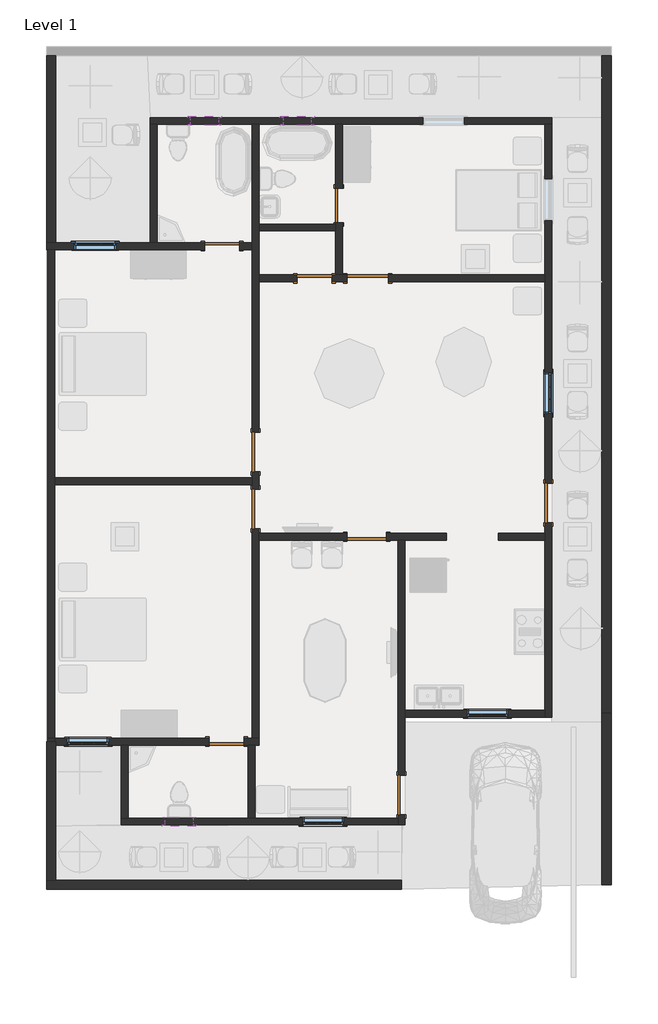
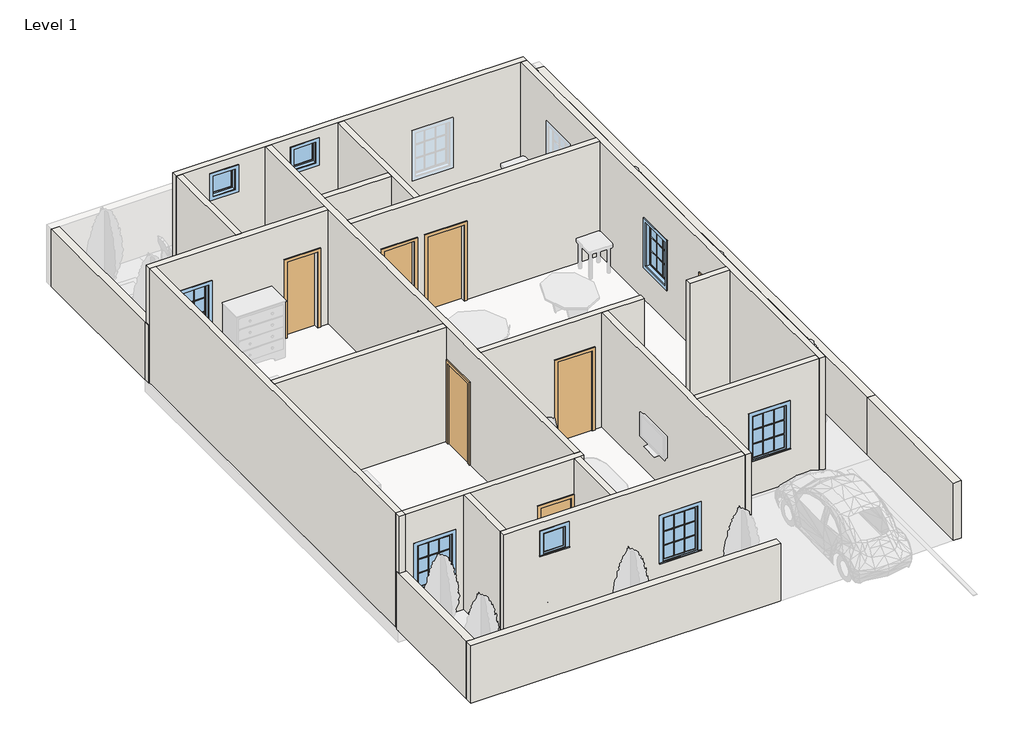
# One storey, part 1 of 2: 24 walls, 10 doors, 8 windows.
"""IFC4 building model written with IfcOpenShell, lengths in millimetres."""

from ifc_helpers import new_model, si_unit, frame, origin, origin_with_axes, place, context, project, spatial, polyline, outline, extrude, faceted_brep, transform, mapped, element, save
from components import door_059fdd7e, door_255cab33, door_99d96fc5, door_b6e9fca3, door_2b0b55a0, window_5c190c7e, window_3d781103

model = new_model("IFC4")

# Units and contexts
model_context = context("Model", 3, world=origin())
ifc_project = project(units=[si_unit("LENGTHUNIT", "METRE", prefix="MILLI")], contexts=[model_context])

# Site, building, storey
site = spatial("IfcSite", under=ifc_project)
building = spatial("IfcBuilding", under=site)
storey = spatial("IfcBuildingStorey", under=building, Name="Level 1", Elevation=0.0)

# Doors
placement = place(None, origin())
door_shape = door_059fdd7e(model_context)
element("IfcDoor", 1, ObjectType="Single-Flush : 30\" x 80\"", at=placement, inside=storey, context=model_context, shape_type="MappedRepresentation", body=[
    mapped(door_shape, transform((-11969.0159934, 7134.0673329, 0.0), x_axis=(1.0, 0.0, 0.0), y_axis=(0.0, 1.0, 0.0), z_axis=(0.0, 0.0, 1.0))),
])
element("IfcDoor", 2, ObjectType="Single-Flush : 30\" x 80\"", at=placement, inside=storey, context=model_context, shape_type="MappedRepresentation", body=[
    mapped(door_shape, transform((-9937.0159934, 6422.8673329, 0.0), x_axis=(1.0, 0.0, 0.0), y_axis=(0.0, 1.0, 0.0), z_axis=(0.0, 0.0, 1.0))),
])
door_2_shape = door_255cab33(model_context)
element("IfcDoor", 3, ObjectType="Single-Flush : 30\" x 80\"", at=placement, inside=storey, context=model_context, shape_type="MappedRepresentation", body=[
    mapped(door_2_shape, transform((-9403.6159934, 8023.0673329, 0.0), x_axis=(0.0, -1.0, 0.0), y_axis=(1.0, 0.0, 0.0), z_axis=(0.0, 0.0, 1.0))),
])
element("IfcDoor", 4, ObjectType="Single-Flush : 30\" x 80\"", at=placement, inside=storey, context=model_context, shape_type="MappedRepresentation", body=[
    mapped(door_2_shape, transform((-11867.4159934, -3737.1326671, 0.0), x_axis=(1.0, 0.0, 0.0), y_axis=(0.0, 1.0, 0.0), z_axis=(0.0, 0.0, 1.0))),
])
door_3_shape = door_99d96fc5(model_context)
element("IfcDoor", 5, ObjectType="Single-Flush : 34\" x 84\"", at=placement, inside=storey, context=model_context, shape_type="MappedRepresentation", body=[
    mapped(door_3_shape, transform((-11232.4159934, 2612.8673329, 0.0), x_axis=(0.0, -1.0, 0.0), y_axis=(1.0, 0.0, 0.0), z_axis=(0.0, 0.0, 1.0))),
])
element("IfcDoor", 6, ObjectType="Single-Flush : 34\" x 84\"", at=placement, inside=storey, context=model_context, shape_type="MappedRepresentation", body=[
    mapped(door_3_shape, transform((-4806.2159934, 1495.2673329, 0.0), x_axis=(0.0, -1.0, 0.0), y_axis=(1.0, 0.0, 0.0), z_axis=(0.0, 0.0, 1.0))),
])
element("IfcDoor", 7, ObjectType="Single-Flush : 34\" x 84\"", at=placement, inside=storey, context=model_context, shape_type="MappedRepresentation", body=[
    mapped(door_3_shape, transform((-8794.0159934, 758.6673329, 0.0), x_axis=(1.0, 0.0, 0.0), y_axis=(0.0, 1.0, 0.0), z_axis=(0.0, 0.0, 1.0))),
])
element("IfcDoor", 8, ObjectType="Single-Flush : 34\" x 84\"", at=placement, inside=storey, context=model_context, shape_type="MappedRepresentation", body=[
    mapped(door_3_shape, transform((-8032.0159934, -4905.5326671, 0.0), x_axis=(0.0, -1.0, 0.0), y_axis=(1.0, 0.0, 0.0), z_axis=(0.0, 0.0, 1.0))),
])
door_4_shape = door_b6e9fca3(model_context)
element("IfcDoor", 9, ObjectType="Single-Flush : 34\" x 84\"", at=placement, inside=storey, context=model_context, shape_type="MappedRepresentation", body=[
    mapped(door_4_shape, transform((-11232.4159934, 1368.2673329, 0.0), x_axis=(0.0, 1.0, 0.0), y_axis=(-1.0, 0.0, 0.0), z_axis=(0.0, 0.0, 1.0))),
])
door_5_shape = door_2b0b55a0(model_context)
element("IfcDoor", 10, ObjectType="Single-Flush : 36\" x 80\"", at=placement, inside=storey, context=model_context, shape_type="MappedRepresentation", body=[
    mapped(door_5_shape, transform((-8768.6159934, 6422.8673329, 0.0), x_axis=(-1.0, 0.0, 0.0), y_axis=(0.0, -1.0, 0.0), z_axis=(0.0, 0.0, 1.0))),
])

# Walls
element("IfcWall", 11, ObjectType="Generic - 8\"", at=placement, inside=storey, context=model_context, shape_type="SweptSolid", body=[
    extrude(outline(polyline([(-3629.9727047, -3120.0940071), (-3629.9727047, 11307.1059929), (-3426.7727047, 11307.1059929), (-3426.7727047, -3120.0940071), (-3629.9727047, -3120.0940071)])), origin_with_axes(), (0.0, 0.0, 1.0), 1524.0),
])
element("IfcWall", 12, ObjectType="Generic - 8\"", at=placement, inside=storey, context=model_context, shape_type="Brep", body=[
    faceted_brep([(-15618.7727047, -6777.6940071, 0.0), (-15618.7727047, -3813.3326671, 0.0), (-15618.7727047, -3737.1326671, 0.0), (-15618.7727047, -3737.1326671, 1524.0), (-15618.7727047, -3813.3326671, 1524.0), (-15618.7727047, -6777.6940071, 1524.0), (-15821.9727047, -6777.6940071, 0.0), (-15821.9727047, -6777.6940071, 1524.0), (-15821.9727047, -3737.1326671, 1524.0), (-15821.9727047, -3737.1326671, 0.0), (-15796.5727047, -3737.1326671, 0.0), (-15644.1727047, -3737.1326671, 0.0), (-15796.5727047, -3737.1326671, 1524.0), (-15644.1727047, -3737.1326671, 1524.0)], [[[0, 1, 2, 3, 4, 5]], [[6, 7, 8, 9]], [[2, 1, 0, 6, 9, 10, 11]], [[3, 2, 11, 10, 9, 8, 12, 13]], [[5, 4, 3, 13, 12, 8, 7]], [[0, 5, 7, 6]]]),
])
element("IfcWall", 13, ObjectType="Generic - 8\"", at=placement, inside=storey, context=model_context, shape_type="Brep", body=[
    faceted_brep([(-15618.7727047, 7210.2673329, 0.0), (-15618.7727047, 11307.1059929, 0.0), (-15618.7727047, 11307.1059929, 1524.0), (-15618.7727047, 7210.2673329, 1524.0), (-15821.9727047, 7210.2673329, 0.0), (-15821.9727047, 7210.2673329, 1524.0), (-15821.9727047, 11307.1059929, 1524.0), (-15821.9727047, 11307.1059929, 0.0), (-15796.5727047, 7210.2673329, 1524.0)], [[[0, 1, 2, 3]], [[4, 5, 6, 7]], [[1, 0, 4, 7]], [[3, 2, 6, 5, 8]], [[2, 1, 7, 6]], [[0, 3, 8, 5, 4]]]),
])
element("IfcWall", 14, ObjectType="Generic - 8\"", at=placement, inside=storey, context=model_context, shape_type="SweptSolid", body=[
    extrude(outline(polyline([(-3629.9727047, -6879.2940071), (-3629.9727047, -3120.0940071), (-3426.7727047, -3120.0940071), (-3426.7727047, -6879.2940071), (-3629.9727047, -6879.2940071)])), origin_with_axes(), (0.0, 0.0, 1.0), 1524.0),
])
element("IfcWall", 15, ObjectType="Generic - 8\"", at=placement, inside=storey, context=model_context, shape_type="Brep", body=[
    faceted_brep([(-8032.0159934, -6777.6940071, 0.0), (-15618.7727047, -6777.6940071, 0.0), (-15821.9727047, -6777.6940071, 0.0), (-15821.9727047, -6777.6940071, 1524.0), (-15618.7727047, -6777.6940071, 1524.0), (-8032.0159934, -6777.6940071, 1524.0), (-8032.0159934, -6980.8940071, 0.0), (-8032.0159934, -6980.8940071, 1524.0), (-15821.9727047, -6980.8940071, 1524.0), (-15821.9727047, -6980.8940071, 0.0)], [[[0, 1, 2, 3, 4, 5]], [[6, 7, 8, 9]], [[2, 1, 0, 6, 9]], [[5, 4, 3, 8, 7]], [[0, 5, 7, 6]], [[3, 2, 9, 8]]]),
])
element("IfcWall", 16, ObjectType="INNER 6\"", at=placement, inside=storey, context=model_context, shape_type="Brep", body=[
    faceted_brep([(-4730.0159934, 9953.4673329, 0.0), (-13543.8159934, 9953.4673329, 0.0), (-13543.8159934, 9953.4673329, 3048.0), (-4730.0159934, 9953.4673329, 3048.0), (-12045.2159934, 9953.4673329, 2768.6), (-12654.8159934, 9953.4673329, 2768.6), (-12654.8159934, 9953.4673329, 2159.0), (-12045.2159934, 9953.4673329, 2159.0), (-10013.2159934, 9953.4673329, 2768.6), (-10622.8159934, 9953.4673329, 2768.6), (-10622.8159934, 9953.4673329, 2159.0), (-10013.2159934, 9953.4673329, 2159.0), (-6647.7159934, 9953.4673329, 2133.6), (-7562.1159934, 9953.4673329, 2133.6), (-7562.1159934, 9953.4673329, 914.4), (-6647.7159934, 9953.4673329, 914.4), (-4730.0159934, 9801.0673329, 0.0), (-4730.0159934, 9801.0673329, 3048.0), (-4882.4159934, 9801.0673329, 3048.0), (-9327.4159934, 9801.0673329, 3048.0), (-9479.8159934, 9801.0673329, 3048.0), (-11156.2159934, 9801.0673329, 3048.0), (-11308.6159934, 9801.0673329, 3048.0), (-13391.4159934, 9801.0673329, 3048.0), (-13543.8159934, 9801.0673329, 3048.0), (-13543.8159934, 9801.0673329, 0.0), (-13391.4159934, 9801.0673329, 0.0), (-11308.6159934, 9801.0673329, 0.0), (-11156.2159934, 9801.0673329, 0.0), (-9479.8159934, 9801.0673329, 0.0), (-9327.4159934, 9801.0673329, 0.0), (-4882.4159934, 9801.0673329, 0.0), (-12045.2159934, 9801.0673329, 2768.6), (-12045.2159934, 9801.0673329, 2159.0), (-12654.8159934, 9801.0673329, 2159.0), (-12654.8159934, 9801.0673329, 2768.6), (-10013.2159934, 9801.0673329, 2768.6), (-10013.2159934, 9801.0673329, 2159.0), (-10622.8159934, 9801.0673329, 2159.0), (-10622.8159934, 9801.0673329, 2768.6), (-6647.7159934, 9801.0673329, 2133.6), (-6647.7159934, 9801.0673329, 914.4), (-7562.1159934, 9801.0673329, 914.4), (-7562.1159934, 9801.0673329, 2133.6)], [[[0, 1, 2, 3], [4, 5, 6, 7], [8, 9, 10, 11], [12, 13, 14, 15]], [[16, 17, 18, 19, 20, 21, 22, 23, 24, 25, 26, 27, 28, 29, 30, 31], [32, 33, 34, 35], [36, 37, 38, 39], [40, 41, 42, 43]], [[1, 0, 16, 31, 30, 29, 28, 27, 26, 25]], [[2, 1, 25, 24]], [[0, 3, 17, 16]], [[33, 32, 4, 7]], [[34, 33, 7, 6]], [[35, 34, 6, 5]], [[32, 35, 5, 4]], [[37, 36, 8, 11]], [[38, 37, 11, 10]], [[39, 38, 10, 9]], [[36, 39, 9, 8]], [[41, 40, 12, 15]], [[42, 41, 15, 14]], [[43, 42, 14, 13]], [[40, 43, 13, 12]], [[3, 2, 24, 23, 22, 21, 20, 19, 18, 17]]]),
])
element("IfcWall", 17, ObjectType="INNER 6\"", at=placement, inside=storey, context=model_context, shape_type="SweptSolid", body=[
    extrude(outline(polyline([(-13543.8159934, 7210.2673329), (-13543.8159934, 9801.0673329), (-13391.4159934, 9801.0673329), (-13391.4159934, 7210.2673329), (-13543.8159934, 7210.2673329)])), origin_with_axes(), (0.0, 0.0, 1.0), 3048.0),
])
element("IfcWall", 18, ObjectType="INNER 6\"", at=placement, inside=storey, context=model_context, shape_type="Brep", body=[
    faceted_brep([(-11308.6159934, 7210.2673329, 0.0), (-11588.0159934, 7210.2673329, 0.0), (-11588.0159934, 7210.2673329, 2032.0), (-12350.0159934, 7210.2673329, 2032.0), (-12350.0159934, 7210.2673329, 0.0), (-13391.4159934, 7210.2673329, 0.0), (-13543.8159934, 7210.2673329, 0.0), (-15618.7727047, 7210.2673329, 0.0), (-15821.9727047, 7210.2673329, 0.0), (-15821.9727047, 7210.2673329, 1524.0), (-15796.5727047, 7210.2673329, 1524.0), (-15796.5727047, 7210.2673329, 3048.0), (-13543.8159934, 7210.2673329, 3048.0), (-13391.4159934, 7210.2673329, 3048.0), (-11308.6159934, 7210.2673329, 3048.0), (-14297.9727047, 7210.2673329, 2133.6), (-15212.3727047, 7210.2673329, 2133.6), (-15212.3727047, 7210.2673329, 914.4), (-14297.9727047, 7210.2673329, 914.4), (-11588.0159934, 7057.8673329, 2032.0), (-11588.0159934, 7057.8673329, 0.0), (-11308.6159934, 7057.8673329, 0.0), (-11308.6159934, 7057.8673329, 3048.0), (-15644.1727047, 7057.8673329, 3048.0), (-15796.5727047, 7057.8673329, 3048.0), (-15796.5727047, 7057.8673329, 1524.0), (-15821.9727047, 7057.8673329, 1524.0), (-15821.9727047, 7057.8673329, 0.0), (-15796.5727047, 7057.8673329, 0.0), (-15644.1727047, 7057.8673329, 0.0), (-12350.0159934, 7057.8673329, 0.0), (-12350.0159934, 7057.8673329, 2032.0), (-14297.9727047, 7057.8673329, 2133.6), (-14297.9727047, 7057.8673329, 914.4), (-15212.3727047, 7057.8673329, 914.4), (-15212.3727047, 7057.8673329, 2133.6)], [[[0, 1, 2, 3, 4, 5, 6, 7, 8, 9, 10, 11, 12, 13, 14], [15, 16, 17, 18]], [[19, 20, 21, 22, 23, 24, 25, 26, 27, 28, 29, 30, 31], [32, 33, 34, 35]], [[21, 20, 1, 0]], [[30, 29, 28, 27, 8, 7, 6, 5, 4]], [[0, 14, 22, 21]], [[2, 1, 20, 19]], [[3, 2, 19, 31]], [[4, 3, 31, 30]], [[33, 32, 15, 18]], [[34, 33, 18, 17]], [[35, 34, 17, 16]], [[32, 35, 16, 15]], [[25, 10, 9, 26]], [[9, 8, 27, 26]], [[11, 10, 25, 24]], [[14, 13, 12, 11, 24, 23, 22]]]),
])
element("IfcWall", 19, ObjectType="INNER 6\"", at=placement, inside=storey, context=model_context, shape_type="Brep", body=[
    faceted_brep([(-4882.4159934, 1063.4673329, 2133.6), (-4882.4159934, 1063.4673329, 0.0), (-4882.4159934, 834.8673329, 0.0), (-4882.4159934, 682.4673329, 0.0), (-4882.4159934, -3051.3326671, 0.0), (-4882.4159934, -3203.7326671, 0.0), (-4882.4159934, -3203.7326671, 3048.0), (-4882.4159934, -3051.3326671, 3048.0), (-4882.4159934, 682.4673329, 3048.0), (-4882.4159934, 834.8673329, 3048.0), (-4882.4159934, 6346.6673329, 3048.0), (-4882.4159934, 6499.0673329, 3048.0), (-4882.4159934, 9801.0673329, 3048.0), (-4882.4159934, 9801.0673329, 0.0), (-4882.4159934, 6499.0673329, 0.0), (-4882.4159934, 6346.6673329, 0.0), (-4882.4159934, 1927.0673329, 0.0), (-4882.4159934, 1927.0673329, 2133.6), (-4882.4159934, 7692.8673329, 2133.6), (-4882.4159934, 7692.8673329, 914.4), (-4882.4159934, 8607.2673329, 914.4), (-4882.4159934, 8607.2673329, 2133.6), (-4882.4159934, 3451.0673329, 2133.6), (-4882.4159934, 3451.0673329, 914.4), (-4882.4159934, 4365.4673329, 914.4), (-4882.4159934, 4365.4673329, 2133.6), (-4730.0159934, -3203.7326671, 0.0), (-4730.0159934, 1063.4673329, 0.0), (-4730.0159934, 1063.4673329, 2133.6), (-4730.0159934, 1927.0673329, 2133.6), (-4730.0159934, 1927.0673329, 0.0), (-4730.0159934, 9801.0673329, 0.0), (-4730.0159934, 9801.0673329, 3048.0), (-4730.0159934, -3203.7326671, 3048.0), (-4730.0159934, 7692.8673329, 2133.6), (-4730.0159934, 8607.2673329, 2133.6), (-4730.0159934, 8607.2673329, 914.4), (-4730.0159934, 7692.8673329, 914.4), (-4730.0159934, 3451.0673329, 2133.6), (-4730.0159934, 4365.4673329, 2133.6), (-4730.0159934, 4365.4673329, 914.4), (-4730.0159934, 3451.0673329, 914.4)], [[[0, 1, 2, 3, 4, 5, 6, 7, 8, 9, 10, 11, 12, 13, 14, 15, 16, 17], [18, 19, 20, 21], [22, 23, 24, 25]], [[26, 27, 28, 29, 30, 31, 32, 33], [34, 35, 36, 37], [38, 39, 40, 41]], [[5, 4, 3, 2, 1, 27, 26]], [[16, 15, 14, 13, 31, 30]], [[13, 12, 32, 31]], [[6, 5, 26, 33]], [[28, 27, 1, 0]], [[29, 28, 0, 17]], [[30, 29, 17, 16]], [[19, 18, 34, 37]], [[20, 19, 37, 36]], [[21, 20, 36, 35]], [[18, 21, 35, 34]], [[23, 22, 38, 41]], [[24, 23, 41, 40]], [[25, 24, 40, 39]], [[22, 25, 39, 38]], [[12, 11, 10, 9, 8, 7, 6, 33, 32]]]),
])
element("IfcWall", 20, ObjectType="INNER 6\"", at=placement, inside=storey, context=model_context, shape_type="SweptSolid", body=[
    extrude(outline(polyline([(0.0, -4882.4159934), (3048.0, -4882.4159934), (3048.0, -7955.8159934), (0.0, -7955.8159934), (0.0, -4882.4159934)]), holes=[polyline([(2133.6, -6596.9159934), (2133.6, -5682.5159934), (914.4, -5682.5159934), (914.4, -6596.9159934), (2133.6, -6596.9159934)])]), frame((0.0, -3203.7326671, 0.0), z_axis=(0.0, 1.0, 0.0), x_axis=(0.0, 0.0, 1.0)), (0.0, 0.0, 1.0), 152.4),
])
element("IfcWall", 21, ObjectType="INNER 6\"", at=placement, inside=storey, context=model_context, shape_type="Brep", body=[
    faceted_brep([(-8108.2159934, -5337.3326671, 2133.6), (-8108.2159934, -5337.3326671, 0.0), (-8108.2159934, -5413.5326671, 0.0), (-8108.2159934, -5565.9326671, 0.0), (-8108.2159934, -5565.9326671, 3048.0), (-8108.2159934, -5413.5326671, 3048.0), (-8108.2159934, 682.4673329, 3048.0), (-8108.2159934, 682.4673329, 0.0), (-8108.2159934, -4473.7326671, 0.0), (-8108.2159934, -4473.7326671, 2133.6), (-7955.8159934, -5565.9326671, 0.0), (-7955.8159934, -5337.3326671, 0.0), (-7955.8159934, -5337.3326671, 2133.6), (-7955.8159934, -4473.7326671, 2133.6), (-7955.8159934, -4473.7326671, 0.0), (-7955.8159934, -3203.7326671, 0.0), (-7955.8159934, -3051.3326671, 0.0), (-7955.8159934, 682.4673329, 0.0), (-7955.8159934, 682.4673329, 3048.0), (-7955.8159934, -3051.3326671, 3048.0), (-7955.8159934, -3203.7326671, 3048.0), (-7955.8159934, -5565.9326671, 3048.0)], [[[0, 1, 2, 3, 4, 5, 6, 7, 8, 9]], [[10, 11, 12, 13, 14, 15, 16, 17, 18, 19, 20, 21]], [[8, 7, 17, 16, 15, 14]], [[3, 2, 1, 11, 10]], [[4, 3, 10, 21]], [[7, 6, 18, 17]], [[12, 11, 1, 0]], [[13, 12, 0, 9]], [[14, 13, 9, 8]], [[6, 5, 4, 21, 20, 19, 18]]]),
])
element("IfcWall", 22, ObjectType="INNER 6\"", at=placement, inside=storey, context=model_context, shape_type="Brep", body=[
    faceted_brep([(-8108.2159934, -5413.5326671, 0.0), (-11246.0185546, -5413.5326671, 0.0), (-11398.4185546, -5413.5326671, 0.0), (-14026.4159934, -5413.5326671, 0.0), (-14178.8159934, -5413.5326671, 0.0), (-14178.8159934, -5413.5326671, 3048.0), (-14026.4159934, -5413.5326671, 3048.0), (-11398.4185546, -5413.5326671, 3048.0), (-11246.0185546, -5413.5326671, 3048.0), (-8108.2159934, -5413.5326671, 3048.0), (-13213.6159934, -5413.5326671, 2768.6), (-13213.6159934, -5413.5326671, 2159.0), (-12604.0159934, -5413.5326671, 2159.0), (-12604.0159934, -5413.5326671, 2768.6), (-10204.6185546, -5413.5326671, 2133.6), (-10204.6185546, -5413.5326671, 914.4), (-9290.2185546, -5413.5326671, 914.4), (-9290.2185546, -5413.5326671, 2133.6), (-8108.2159934, -5565.9326671, 0.0), (-8108.2159934, -5565.9326671, 3048.0), (-14178.8159934, -5565.9326671, 3048.0), (-14178.8159934, -5565.9326671, 0.0), (-13213.6159934, -5565.9326671, 2768.6), (-12604.0159934, -5565.9326671, 2768.6), (-12604.0159934, -5565.9326671, 2159.0), (-13213.6159934, -5565.9326671, 2159.0), (-10204.6185546, -5565.9326671, 2133.6), (-9290.2185546, -5565.9326671, 2133.6), (-9290.2185546, -5565.9326671, 914.4), (-10204.6185546, -5565.9326671, 914.4)], [[[0, 1, 2, 3, 4, 5, 6, 7, 8, 9], [10, 11, 12, 13], [14, 15, 16, 17]], [[18, 19, 20, 21], [22, 23, 24, 25], [26, 27, 28, 29]], [[4, 3, 2, 1, 0, 18, 21]], [[0, 9, 19, 18]], [[5, 4, 21, 20]], [[11, 10, 22, 25]], [[12, 11, 25, 24]], [[13, 12, 24, 23]], [[10, 13, 23, 22]], [[15, 14, 26, 29]], [[16, 15, 29, 28]], [[17, 16, 28, 27]], [[14, 17, 27, 26]], [[9, 8, 7, 6, 5, 20, 19]]]),
])
element("IfcWall", 23, ObjectType="INNER 6\"", at=placement, inside=storey, context=model_context, shape_type="SweptSolid", body=[
    extrude(outline(polyline([(-14026.4159934, -3813.3326671), (-14026.4159934, -5413.5326671), (-14178.8159934, -5413.5326671), (-14178.8159934, -3813.3326671), (-14026.4159934, -3813.3326671)])), origin_with_axes(), (0.0, 0.0, 1.0), 3048.0),
])
element("IfcWall", 24, ObjectType="INNER 6\"", at=placement, inside=storey, context=model_context, shape_type="Brep", body=[
    faceted_brep([(-11156.2159934, -3660.9326671, 0.0), (-11308.6159934, -3660.9326671, 0.0), (-11486.4159934, -3660.9326671, 0.0), (-11486.4159934, -3660.9326671, 2032.0), (-12248.4159934, -3660.9326671, 2032.0), (-12248.4159934, -3660.9326671, 0.0), (-15644.1727047, -3660.9326671, 0.0), (-15644.1727047, -3660.9326671, 1524.0), (-15644.1727047, -3660.9326671, 3048.0), (-11308.6159934, -3660.9326671, 3048.0), (-11156.2159934, -3660.9326671, 3048.0), (-15368.694349, -3660.9326671, 2133.6), (-15368.694349, -3660.9326671, 914.4), (-14454.294349, -3660.9326671, 914.4), (-14454.294349, -3660.9326671, 2133.6), (-11486.4159934, -3813.3326671, 2032.0), (-11486.4159934, -3813.3326671, 0.0), (-11398.4185546, -3813.3326671, 0.0), (-11246.0185546, -3813.3326671, 0.0), (-11156.2159934, -3813.3326671, 0.0), (-11156.2159934, -3813.3326671, 3048.0), (-11246.0185546, -3813.3326671, 3048.0), (-11398.4185546, -3813.3326671, 3048.0), (-14026.4159934, -3813.3326671, 3048.0), (-14178.8159934, -3813.3326671, 3048.0), (-15644.1727047, -3813.3326671, 3048.0), (-15644.1727047, -3813.3326671, 1524.0), (-15618.7727047, -3813.3326671, 1524.0), (-15618.7727047, -3813.3326671, 0.0), (-14178.8159934, -3813.3326671, 0.0), (-14026.4159934, -3813.3326671, 0.0), (-12248.4159934, -3813.3326671, 0.0), (-12248.4159934, -3813.3326671, 2032.0), (-15368.694349, -3813.3326671, 2133.6), (-14454.294349, -3813.3326671, 2133.6), (-14454.294349, -3813.3326671, 914.4), (-15368.694349, -3813.3326671, 914.4), (-15618.7727047, -3737.1326671, 0.0), (-15644.1727047, -3737.1326671, 0.0), (-15644.1727047, -3737.1326671, 1524.0), (-15618.7727047, -3737.1326671, 1524.0)], [[[0, 1, 2, 3, 4, 5, 6, 7, 8, 9, 10], [11, 12, 13, 14]], [[15, 16, 17, 18, 19, 20, 21, 22, 23, 24, 25, 26, 27, 28, 29, 30, 31, 32], [33, 34, 35, 36]], [[19, 18, 17, 16, 2, 1, 0]], [[31, 30, 29, 28, 37, 38, 6, 5]], [[0, 10, 20, 19]], [[26, 39, 40, 27]], [[7, 6, 38, 39]], [[8, 7, 39, 26, 25]], [[3, 2, 16, 15]], [[4, 3, 15, 32]], [[5, 4, 32, 31]], [[12, 11, 33, 36]], [[13, 12, 36, 35]], [[14, 13, 35, 34]], [[11, 14, 34, 33]], [[10, 9, 8, 25, 24, 23, 22, 21, 20]], [[38, 37, 40, 39]], [[37, 28, 27, 40]]]),
])
element("IfcWall", 25, ObjectType="INNER 6\"", at=placement, inside=storey, context=model_context, shape_type="Brep", body=[
    faceted_brep([(-11156.2159934, 1800.0673329, 2133.6), (-11156.2159934, 1800.0673329, 0.0), (-11156.2159934, 2181.0673329, 0.0), (-11156.2159934, 2181.0673329, 2133.6), (-11156.2159934, 3044.6673329, 2133.6), (-11156.2159934, 3044.6673329, 0.0), (-11156.2159934, 6346.6673329, 0.0), (-11156.2159934, 6499.0673329, 0.0), (-11156.2159934, 7464.2673329, 0.0), (-11156.2159934, 7616.6673329, 0.0), (-11156.2159934, 9801.0673329, 0.0), (-11156.2159934, 9801.0673329, 3048.0), (-11156.2159934, 7616.6673329, 3048.0), (-11156.2159934, 7464.2673329, 3048.0), (-11156.2159934, 6499.0673329, 3048.0), (-11156.2159934, 6346.6673329, 3048.0), (-11156.2159934, 834.8673329, 3048.0), (-11156.2159934, 682.4673329, 3048.0), (-11156.2159934, -3660.9326671, 3048.0), (-11156.2159934, -3660.9326671, 0.0), (-11156.2159934, 682.4673329, 0.0), (-11156.2159934, 834.8673329, 0.0), (-11156.2159934, 936.4673329, 0.0), (-11156.2159934, 936.4673329, 2133.6), (-11308.6159934, 2181.0673329, 0.0), (-11308.6159934, 2054.0673329, 0.0), (-11308.6159934, 1901.6673329, 0.0), (-11308.6159934, 1800.0673329, 0.0), (-11308.6159934, 1800.0673329, 2133.6), (-11308.6159934, 936.4673329, 2133.6), (-11308.6159934, 936.4673329, 0.0), (-11308.6159934, -3660.9326671, 0.0), (-11308.6159934, -3660.9326671, 3048.0), (-11308.6159934, 1901.6673329, 3048.0), (-11308.6159934, 2054.0673329, 3048.0), (-11308.6159934, 7057.8673329, 3048.0), (-11308.6159934, 7210.2673329, 3048.0), (-11308.6159934, 9801.0673329, 3048.0), (-11308.6159934, 9801.0673329, 0.0), (-11308.6159934, 7210.2673329, 0.0), (-11308.6159934, 7057.8673329, 0.0), (-11308.6159934, 3044.6673329, 0.0), (-11308.6159934, 3044.6673329, 2133.6), (-11308.6159934, 2181.0673329, 2133.6)], [[[0, 1, 2, 3, 4, 5, 6, 7, 8, 9, 10, 11, 12, 13, 14, 15, 16, 17, 18, 19, 20, 21, 22, 23]], [[24, 25, 26, 27, 28, 29, 30, 31, 32, 33, 34, 35, 36, 37, 38, 39, 40, 41, 42, 43]], [[41, 40, 39, 38, 10, 9, 8, 7, 6, 5]], [[2, 1, 27, 26, 25, 24]], [[22, 21, 20, 19, 31, 30]], [[11, 10, 38, 37]], [[19, 18, 32, 31]], [[3, 2, 24, 43]], [[4, 3, 43, 42]], [[5, 4, 42, 41]], [[28, 27, 1, 0]], [[29, 28, 0, 23]], [[30, 29, 23, 22]], [[18, 17, 16, 15, 14, 13, 12, 11, 37, 36, 35, 34, 33, 32]]]),
])
element("IfcWall", 26, ObjectType="INNER 6\"", at=placement, inside=storey, context=model_context, shape_type="SweptSolid", body=[
    extrude(outline(polyline([(-11398.4185546, -5413.5326671), (-11398.4185546, -3813.3326671), (-11246.0185546, -3813.3326671), (-11246.0185546, -5413.5326671), (-11398.4185546, -5413.5326671)])), origin_with_axes(), (0.0, 0.0, 1.0), 3048.0),
])
element("IfcWall", 27, ObjectType="INNER 6\"", at=placement, inside=storey, context=model_context, shape_type="SweptSolid", body=[
    extrude(outline(polyline([(-5898.4159934, 834.8673329), (-4882.4159934, 834.8673329), (-4882.4159934, 682.4673329), (-5898.4159934, 682.4673329), (-5898.4159934, 834.8673329)])), origin_with_axes(), (0.0, 0.0, 1.0), 3048.0),
])
element("IfcWall", 28, ObjectType="INNER 6\"", at=placement, inside=storey, context=model_context, shape_type="Brep", body=[
    faceted_brep([(-9556.0159934, 6346.6673329, 0.0), (-9225.8159934, 6346.6673329, 0.0), (-9225.8159934, 6346.6673329, 2032.0), (-8311.4159934, 6346.6673329, 2032.0), (-8311.4159934, 6346.6673329, 0.0), (-4882.4159934, 6346.6673329, 0.0), (-4882.4159934, 6346.6673329, 3048.0), (-11156.2159934, 6346.6673329, 3048.0), (-11156.2159934, 6346.6673329, 0.0), (-10318.0159934, 6346.6673329, 0.0), (-10318.0159934, 6346.6673329, 2032.0), (-9556.0159934, 6346.6673329, 2032.0), (-9225.8159934, 6499.0673329, 2032.0), (-9225.8159934, 6499.0673329, 0.0), (-9327.4159934, 6499.0673329, 0.0), (-9479.8159934, 6499.0673329, 0.0), (-9556.0159934, 6499.0673329, 0.0), (-9556.0159934, 6499.0673329, 2032.0), (-10318.0159934, 6499.0673329, 2032.0), (-10318.0159934, 6499.0673329, 0.0), (-11156.2159934, 6499.0673329, 0.0), (-11156.2159934, 6499.0673329, 3048.0), (-9479.8159934, 6499.0673329, 3048.0), (-9327.4159934, 6499.0673329, 3048.0), (-4882.4159934, 6499.0673329, 3048.0), (-4882.4159934, 6499.0673329, 0.0), (-8311.4159934, 6499.0673329, 0.0), (-8311.4159934, 6499.0673329, 2032.0)], [[[0, 1, 2, 3, 4, 5, 6, 7, 8, 9, 10, 11]], [[12, 13, 14, 15, 16, 17, 18, 19, 20, 21, 22, 23, 24, 25, 26, 27]], [[9, 8, 20, 19]], [[26, 25, 5, 4]], [[16, 15, 14, 13, 1, 0]], [[6, 5, 25, 24]], [[8, 7, 21, 20]], [[17, 16, 0, 11]], [[18, 17, 11, 10]], [[19, 18, 10, 9]], [[2, 1, 13, 12]], [[3, 2, 12, 27]], [[4, 3, 27, 26]], [[7, 6, 24, 23, 22, 21]]]),
])
element("IfcWall", 29, ObjectType="INNER 6\"", at=placement, inside=storey, context=model_context, shape_type="Brep", body=[
    faceted_brep([(-15644.1727047, -3737.1326671, 0.0), (-15644.1727047, -3660.9326671, 0.0), (-15644.1727047, -3660.9326671, 1524.0), (-15644.1727047, -3660.9326671, 3048.0), (-15644.1727047, -3813.3326671, 3048.0), (-15644.1727047, -3813.3326671, 1524.0), (-15644.1727047, -3737.1326671, 1524.0), (-15796.5727047, -3737.1326671, 0.0), (-15796.5727047, -3737.1326671, 1524.0), (-15796.5727047, -3813.3326671, 1524.0), (-15796.5727047, -3813.3326671, 3048.0), (-15796.5727047, -3660.9326671, 3048.0), (-15796.5727047, -3660.9326671, 0.0)], [[[0, 1, 2, 3, 4, 5, 6]], [[7, 8, 9, 10, 11, 12]], [[1, 0, 7, 12]], [[3, 2, 1, 12, 11]], [[0, 6, 8, 7]], [[5, 9, 8, 6]], [[5, 4, 10, 9]], [[4, 3, 11, 10]]]),
])
element("IfcWall", 30, ObjectType="INNER 6\"", at=placement, inside=storey, context=model_context, shape_type="SweptSolid", body=[
    extrude(outline(polyline([(-15644.1727047, 2054.0673329), (-11308.6159934, 2054.0673329), (-11308.6159934, 1901.6673329), (-15644.1727047, 1901.6673329), (-15644.1727047, 2054.0673329)])), origin_with_axes(), (0.0, 0.0, 1.0), 3048.0),
])
element("IfcWall", 31, ObjectType="INNER 6\"", at=placement, inside=storey, context=model_context, shape_type="Brep", body=[
    faceted_brep([(-9479.8159934, 7642.0673329, 2032.0), (-9479.8159934, 7642.0673329, 0.0), (-9479.8159934, 7616.6673329, 0.0), (-9479.8159934, 7464.2673329, 0.0), (-9479.8159934, 6499.0673329, 0.0), (-9479.8159934, 6499.0673329, 3048.0), (-9479.8159934, 7464.2673329, 3048.0), (-9479.8159934, 7616.6673329, 3048.0), (-9479.8159934, 9801.0673329, 3048.0), (-9479.8159934, 9801.0673329, 0.0), (-9479.8159934, 8404.0673329, 0.0), (-9479.8159934, 8404.0673329, 2032.0), (-9327.4159934, 6499.0673329, 0.0), (-9327.4159934, 7642.0673329, 0.0), (-9327.4159934, 7642.0673329, 2032.0), (-9327.4159934, 8404.0673329, 2032.0), (-9327.4159934, 8404.0673329, 0.0), (-9327.4159934, 9801.0673329, 0.0), (-9327.4159934, 9801.0673329, 3048.0), (-9327.4159934, 6499.0673329, 3048.0)], [[[0, 1, 2, 3, 4, 5, 6, 7, 8, 9, 10, 11]], [[12, 13, 14, 15, 16, 17, 18, 19]], [[10, 9, 17, 16]], [[4, 3, 2, 1, 13, 12]], [[9, 8, 18, 17]], [[5, 4, 12, 19]], [[14, 13, 1, 0]], [[15, 14, 0, 11]], [[16, 15, 11, 10]], [[8, 7, 6, 5, 19, 18]]]),
])
element("IfcWall", 32, ObjectType="INNER 6\"", at=placement, inside=storey, context=model_context, shape_type="SweptSolid", body=[
    extrude(outline(polyline([(-11156.2159934, 7616.6673329), (-9479.8159934, 7616.6673329), (-9479.8159934, 7464.2673329), (-11156.2159934, 7464.2673329), (-11156.2159934, 7616.6673329)])), origin_with_axes(), (0.0, 0.0, 1.0), 3048.0),
])
element("IfcWall", 33, ObjectType="INNER 6\"", at=placement, inside=storey, context=model_context, shape_type="Brep", body=[
    faceted_brep([(-7041.4159934, 834.8673329, 0.0), (-8362.2159934, 834.8673329, 0.0), (-8362.2159934, 834.8673329, 2133.6), (-9225.8159934, 834.8673329, 2133.6), (-9225.8159934, 834.8673329, 0.0), (-11156.2159934, 834.8673329, 0.0), (-11156.2159934, 834.8673329, 3048.0), (-7041.4159934, 834.8673329, 3048.0), (-8362.2159934, 682.4673329, 2133.6), (-8362.2159934, 682.4673329, 0.0), (-8108.2159934, 682.4673329, 0.0), (-7955.8159934, 682.4673329, 0.0), (-7041.4159934, 682.4673329, 0.0), (-7041.4159934, 682.4673329, 3048.0), (-7955.8159934, 682.4673329, 3048.0), (-8108.2159934, 682.4673329, 3048.0), (-11156.2159934, 682.4673329, 3048.0), (-11156.2159934, 682.4673329, 0.0), (-9225.8159934, 682.4673329, 0.0), (-9225.8159934, 682.4673329, 2133.6)], [[[0, 1, 2, 3, 4, 5, 6, 7]], [[8, 9, 10, 11, 12, 13, 14, 15, 16, 17, 18, 19]], [[18, 17, 5, 4]], [[12, 11, 10, 9, 1, 0]], [[0, 7, 13, 12]], [[6, 5, 17, 16]], [[4, 3, 19, 18]], [[3, 2, 8, 19]], [[2, 1, 9, 8]], [[7, 6, 16, 15, 14, 13]]]),
])
element("IfcWall", 34, ObjectType="INNER 6\"", at=placement, inside=storey, context=model_context, shape_type="Brep", body=[
    faceted_brep([(-15796.5727047, 7057.8673329, 0.0), (-15796.5727047, -3660.9326671, 0.0), (-15796.5727047, -3660.9326671, 3048.0), (-15796.5727047, 7057.8673329, 3048.0), (-15796.5727047, 7057.8673329, 1524.0), (-15644.1727047, 7057.8673329, 0.0), (-15644.1727047, 7057.8673329, 3048.0), (-15644.1727047, 2054.0673329, 3048.0), (-15644.1727047, 1901.6673329, 3048.0), (-15644.1727047, -3660.9326671, 3048.0), (-15644.1727047, -3660.9326671, 0.0), (-15644.1727047, 1901.6673329, 0.0), (-15644.1727047, 2054.0673329, 0.0)], [[[0, 1, 2, 3, 4]], [[5, 6, 7, 8, 9, 10, 11, 12]], [[1, 0, 5, 12, 11, 10]], [[2, 1, 10, 9]], [[0, 4, 3, 6, 5]], [[3, 2, 9, 8, 7, 6]]]),
])

# Windows
window_shape = window_5c190c7e(model_context)
element("IfcWindow", 35, ObjectType="Casement 3x3 with Trim : 36\" x 48\"", at=placement, inside=storey, context=model_context, shape_type="MappedRepresentation", body=[
    mapped(window_shape, transform((-14755.1727047, 7134.0673329, 0.0), x_axis=(1.0, 0.0, 0.0), y_axis=(0.0, 1.0, 0.0), z_axis=(0.0, 0.0, 1.0))),
])
element("IfcWindow", 36, ObjectType="Casement 3x3 with Trim : 36\" x 48\"", at=placement, inside=storey, context=model_context, shape_type="MappedRepresentation", body=[
    mapped(window_shape, transform((-4806.2159934, 3908.2673329, 0.0), x_axis=(0.0, -1.0, 0.0), y_axis=(1.0, 0.0, 0.0), z_axis=(0.0, 0.0, 1.0))),
])
element("IfcWindow", 37, ObjectType="Casement 3x3 with Trim : 36\" x 48\"", at=placement, inside=storey, context=model_context, shape_type="MappedRepresentation", body=[
    mapped(window_shape, transform((-6139.7159934, -3127.5326671, 0.0), x_axis=(-1.0, 0.0, 0.0), y_axis=(0.0, -1.0, 0.0), z_axis=(0.0, 0.0, 1.0))),
])
element("IfcWindow", 38, ObjectType="Casement 3x3 with Trim : 36\" x 48\"", at=placement, inside=storey, context=model_context, shape_type="MappedRepresentation", body=[
    mapped(window_shape, transform((-9747.4185546, -5489.7326671, 0.0), x_axis=(-1.0, 0.0, 0.0), y_axis=(0.0, -1.0, 0.0), z_axis=(0.0, 0.0, 1.0))),
])
element("IfcWindow", 39, ObjectType="Casement 3x3 with Trim : 36\" x 48\"", at=placement, inside=storey, context=model_context, shape_type="MappedRepresentation", body=[
    mapped(window_shape, transform((-14911.494349, -3737.1326671, 0.0), x_axis=(-1.0, 0.0, 0.0), y_axis=(0.0, -1.0, 0.0), z_axis=(0.0, 0.0, 1.0))),
])
window_2_shape = window_3d781103(model_context)
element("IfcWindow", 40, ObjectType="Transom with Trim : 24\" x 24\"", at=placement, inside=storey, context=model_context, shape_type="MappedRepresentation", body=[
    mapped(window_2_shape, transform((-12311.9159934, 9877.2673329, 0.0), x_axis=(1.0, 0.0, 0.0), y_axis=(0.0, 1.0, 0.0), z_axis=(0.0, 0.0, 1.0))),
])
element("IfcWindow", 41, ObjectType="Transom with Trim : 24\" x 24\"", at=placement, inside=storey, context=model_context, shape_type="MappedRepresentation", body=[
    mapped(window_2_shape, transform((-10279.9159934, 9877.2673329, 0.0), x_axis=(1.0, 0.0, 0.0), y_axis=(0.0, 1.0, 0.0), z_axis=(0.0, 0.0, 1.0))),
])
element("IfcWindow", 42, ObjectType="Transom with Trim : 24\" x 24\"", at=placement, inside=storey, context=model_context, shape_type="MappedRepresentation", body=[
    mapped(window_2_shape, transform((-12946.9159934, -5489.7326671, 0.0), x_axis=(-1.0, 0.0, 0.0), y_axis=(0.0, -1.0, 0.0), z_axis=(0.0, 0.0, 1.0))),
])

save(model, "model.ifc")

# Revit data of these elements
# Type "Single-Flush : 30\" x 80\""
#   Type Mark = "5"
#   Construction Type Id = "MDOOR"
#   Assembly Code = "C1020"
#   Analytic Construction = "Metal"
#   Thickness = 0' - 2"
#   Heat Transfer Coefficient (U) = 0.651978 BTU/(h·ft²·°F)
#   Height = 6' - 8"
#   Trim Projection Ext = 0' - 1"
#   Trim Projection Int = 0' - 1"
#   Trim Width = 0' - 3"
#   Width = 2' - 6"
#   Define Thermal Properties by = 1
#   Door Material = Door - Panel
#   Frame Material = Door - Frame
#   Visual Light Transmittance = 0
#   Solar Heat Gain Coefficient = 0
#   Function = (empty or 0)
#   Wall Closure = (empty or 0)
# Type "Single-Flush : 34\" x 84\""
#   Type Mark = "2"
#   Construction Type Id = "MDOOR"
#   Assembly Code = "C1020"
#   Analytic Construction = "Metal"
#   Thickness = 0' - 2"
#   Heat Transfer Coefficient (U) = 0.651978 BTU/(h·ft²·°F)
#   Height = 7' - 0"
#   Trim Projection Ext = 0' - 1"
#   Trim Projection Int = 0' - 1"
#   Trim Width = 0' - 3"
#   Width = 2' - 10"
#   Define Thermal Properties by = 1
#   Door Material = Door - Panel
#   Frame Material = Door - Frame
#   Visual Light Transmittance = 0
#   Solar Heat Gain Coefficient = 0
#   Function = (empty or 0)
#   Wall Closure = (empty or 0)
# Type "Single-Flush : 36\" x 80\""
#   Type Mark = "6"
#   Construction Type Id = "MDOOR"
#   Assembly Code = "C1020"
#   Analytic Construction = "Metal"
#   Thickness = 0' - 2"
#   Heat Transfer Coefficient (U) = 0.651978 BTU/(h·ft²·°F)
#   Height = 6' - 8"
#   Trim Projection Ext = 0' - 1"
#   Trim Projection Int = 0' - 1"
#   Trim Width = 0' - 3"
#   Width = 3' - 0"
#   Define Thermal Properties by = 1
#   Door Material = Door - Panel
#   Frame Material = Door - Frame
#   Visual Light Transmittance = 0
#   Solar Heat Gain Coefficient = 0
#   Function = (empty or 0)
#   Wall Closure = (empty or 0)
# Type "Generic - 8\""
#   Assembly Code = "B2010"
#   Layers, outside or top first: 0' - 8" "Birch" (function 1)
# Type "INNER 6\""
#   Assembly Code = "B2010"
#   Layers, outside or top first: 0' - 6" "Brick, Common" (function 1)
# Type "Casement 3x3 with Trim : 36\" x 48\""
#   Type Mark = "20"
#   Construction Type Id = "GSP4R"
#   Assembly Code = "B2020100"
#   Analytic Construction = "1/8 in Pilkington single glazing"
#   Visual Light Transmittance = 0.9
#   Solar Heat Gain Coefficient = 0.78
#   Heat Transfer Coefficient (U) = 0.6496 BTU/(h·ft²·°F)
#   Height = 4' - 0"
#   Default Sill Height = 3' - 0"
#   Trim Projection - Ext. = 0' - 0 1/2"
#   Trim Projection - Int. = 0' - 0 3/4"
#   Trim Width - Exterior = 0' - 3 1/2"
#   Trim Width - Interior = 0' - 3 1/2"
#   Width = 3' - 0"
#   Window Inset = 0' - 0 3/4"
#   Define Thermal Properties by = 1
#   Glass Pane Material = Glass
#   Sash Material = Sash
#   Trim Exterior Material = Trim
#   Trim Interior Material = Trim
#   Wall Closure = (empty or 0)
# Type "Transom with Trim : 24\" x 24\""
#   Type Mark = "10"
#   Construction Type Id = "GSP4R"
#   Assembly Code = "B2020100"
#   Analytic Construction = "1/8 in Pilkington single glazing"
#   Visual Light Transmittance = 0.9
#   Solar Heat Gain Coefficient = 0.78
#   Heat Transfer Coefficient (U) = 0.6496 BTU/(h·ft²·°F)
#   Height = 2' - 0"
#   Default Sill Height = 7' - 1"
#   Trim Projection - Ext. = 0' - 0 1/2"
#   Trim Projection - Int. = 0' - 0 3/4"
#   Trim Width - Exterior = 0' - 3 1/2"
#   Trim Width - Interior = 0' - 3 1/2"
#   Width = 2' - 0"
#   Window Inset = 0' - 0 3/4"
#   Define Thermal Properties by = 1
#   Glass Pane Material = Glass
#   Sash Material = Sash
#   Trim Exterior Material = Trim
#   Trim Interior Material = Trim
#   Wall Closure = (empty or 0)
# Elements 1, 2, 3, 4 (IfcDoor, "Single-Flush : 30\" x 80\"")
#   Phase Created = New Construction
#   Materials on its faces: "Door - Frame", "Door - Panel"
# Elements 5, 6, 7, 8, 9 (IfcDoor, "Single-Flush : 34\" x 84\"")
#   Phase Created = New Construction
#   Materials on its faces: "Door - Frame", "Door - Panel"
# Element 10 (IfcDoor, "Single-Flush : 36\" x 80\"")
#   Phase Created = New Construction
#   Materials on its faces: "Door - Frame", "Door - Panel"
# Elements 11, 12, 13, 14, 15 (IfcWall, "Generic - 8\"")
#   Top Offset = 0' - 0"
#   Base Offset = 0' - 0"
#   Unconnected Height = 5' - 0"
#   wall height = 5' - 0"
#   Phase Created = New Construction
#   Base Constraint = Level 1
#   Materials on its faces: "Birch"
# Elements 16, 17, 19, 20, 21, 22, 23, 24, 25, 26, 27, 28, 29, 30, 31, 32, 33, 34 (IfcWall, "INNER 6\"")
#   Top Offset = 0' - 0"
#   Base Offset = 0' - 0"
#   Unconnected Height = 10' - 0"
#   wall height = 10' - 0"
#   Phase Created = New Construction
#   Base Constraint = Level 1
#   Materials on its faces: "Brick, Common"
# Element 18 (IfcWall, "INNER 6\"")
#   Top Offset = 0' - 0"
#   Base Offset = 0' - 0"
#   Unconnected Height = 10' - 0"
#   wall height = 10' - 0"
#   Phase Created = New Construction
#   Base Constraint = Level 1
#   Materials on its faces: "Brick, Common", "Birch"
# Element 35 (IfcWindow, "Casement 3x3 with Trim : 36\" x 48\"")
#   Mark = "4"
#   Phase Created = New Construction
#   Materials on its faces: "Sash", "Glass", "Trim"
# Element 36 (IfcWindow, "Casement 3x3 with Trim : 36\" x 48\"")
#   Mark = "7"
#   Phase Created = New Construction
#   Materials on its faces: "Sash", "Glass", "Trim"
# Element 37 (IfcWindow, "Casement 3x3 with Trim : 36\" x 48\"")
#   Mark = "8"
#   Phase Created = New Construction
#   Materials on its faces: "Sash", "Glass", "Trim"
# Element 38 (IfcWindow, "Casement 3x3 with Trim : 36\" x 48\"")
#   Mark = "9"
#   Phase Created = New Construction
#   Materials on its faces: "Sash", "Glass", "Trim"
# Element 39 (IfcWindow, "Casement 3x3 with Trim : 36\" x 48\"")
#   Mark = "10"
#   Phase Created = New Construction
#   Materials on its faces: "Sash", "Glass", "Trim"
# Element 40 (IfcWindow, "Transom with Trim : 24\" x 24\"")
#   Mark = "1"
#   Phase Created = New Construction
#   Materials on its faces: "Sash", "Trim", "Glass"
# Element 41 (IfcWindow, "Transom with Trim : 24\" x 24\"")
#   Mark = "2"
#   Phase Created = New Construction
#   Materials on its faces: "Sash", "Trim", "Glass"
# Element 42 (IfcWindow, "Transom with Trim : 24\" x 24\"")
#   Mark = "3"
#   Phase Created = New Construction
#   Materials on its faces: "Sash", "Trim", "Glass"
# Materials
#   "Door - Panel": class "Wood", colour RGB 210 159 95, transparency 0
#   "Door - Frame": colour RGB 118 70 51, transparency 0
#   "Birch": class "Wood", colour RGB 224 178 126, transparency 0, Description = "Betula Alleghaniensis", Cost = 0
#   "Brick, Common": class "Masonry", colour RGB 170 98 104, transparency 0, Description = "Common brick", Cost = 0
#   "Glass": class "Glass", colour RGB 0 128 192, transparency 0.75, Description = "Soda Lime Glass", Cost = 0
#   "Sash": class "Wood", colour RGB 224 178 126, transparency 0
#   "Trim": class "Wood", colour RGB 224 178 126, transparency 0
# Room at (-10383.006, 6847.719) mm, phase "New Construction", upper level "Level 1", upper offset 10' - 0", lower offset 0' - 0"
#   Number = "5"
#   Name = "STORE"
# Room at (-13345.975, 4265.674) mm, phase "New Construction", upper level "Level 1", upper offset 10' - 0", lower offset 0' - 0"
#   Number = "6"
#   Name = "BEDROOM"
# Room at (-6854.668, 8585.169) mm, phase "New Construction", upper level "Level 1", upper offset 10' - 0", lower offset 0' - 0"
#   Number = "4"
#   Name = "BEDROOM"
# Room at (-9460.843, 11070.689) mm, phase "New Construction", upper level "Level 1", upper offset 10' - 0", lower offset 0' - 0"
#   Number = "1"
#   Name = "WIDE PASSAGE"
# Room at (-12211.806, 8585.169) mm, phase "New Construction", upper level "Level 1", upper offset 10' - 0", lower offset 0' - 0"
#   Number = "2"
# Room at (-10383.006, 8585.169) mm, phase "New Construction", upper level "Level 1", upper offset 10' - 0", lower offset 0' - 0"
#   Number = "3"
# Room at (-8133.624, 3493.474) mm, phase "New Construction", upper level "Level 1", upper offset 10' - 0", lower offset 0' - 0"
#   Number = "7"
#   Name = "LOUNGE"
# Room at (-12959.875, -729.496) mm, phase "New Construction", upper level "Level 1", upper offset 10' - 0", lower offset 0' - 0"
#   Number = "8"
#   Name = "BEDROOM"
# Room at (-9629.762, -1991.651) mm, phase "New Construction", upper level "Level 1", upper offset 10' - 0", lower offset 0' - 0"
#   Number = "9"
# Room at (-12959.875, -4735.284) mm, phase "New Construction", upper level "Level 1", upper offset 10' - 0", lower offset 0' - 0"
#   Number = "10"
# Room at (-12211.806, -6496.866) mm, phase "New Construction", upper level "Level 1", upper offset 10' - 0", lower offset 0' - 0"
#   Number = "11"
#   Name = "LAWN"
# Room at (-6304.824, -1260.383) mm, phase "New Construction", upper level "Level 1", upper offset 10' - 0", lower offset 0' - 0"
#   Number = "12"
#   Name = "KITCHEN"
# Room at (-5817.023, -5997.44) mm, phase "New Construction", upper level "Level 1", upper offset 10' - 0", lower offset 0' - 0"
#   Number = "13"
#   Name = "PARKING"
# Room at (-3988.223, 1345.792) mm, phase "New Construction", upper level "Level 1", upper offset 10' - 0", lower offset 0' - 0"
#   Number = "14"
#   Name = "WIDE PASSAGE"
